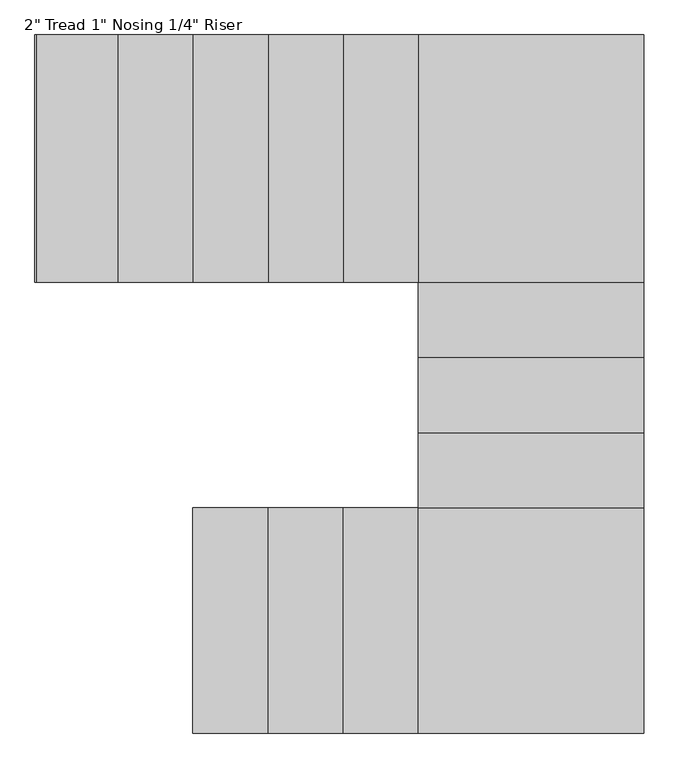
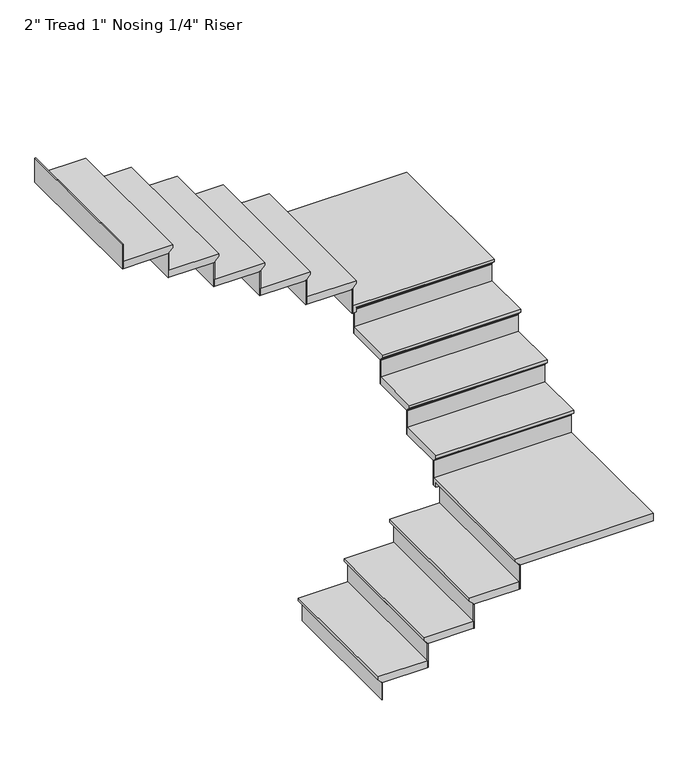
"""IFC4 building model written with IfcOpenShell, lengths in millimetres: stair flight geometry."""

from ifc_helpers import new_model, si_unit, origin, place, context, project, spatial, faceted_brep, source, transform, mapped, element, save


def stair_flight_3451e034(model_context):
    return source(origin(), model_context, "Body", "Brep", [
        faceted_brep([(938.5174794, -182.0870507, 3350.6833333), (938.5174794, -182.0870507, 3369.7333333), (938.5174794, 732.3129493, 3369.7333333), (938.5174794, 732.3129493, 3350.6833333), (963.9174794, -182.0870507, 3325.2833333), (963.9174794, 732.3129493, 3325.2833333), (1268.7174794, -182.0870507, 3369.7333333), (1268.7174794, 732.3129493, 3369.7333333), (963.9174794, 732.3129493, 3318.9333333), (1268.7174794, 732.3129493, 3318.9333333), (1268.7174794, -182.0870507, 3318.9333333), (963.9174794, -182.0870507, 3318.9333333)], [[[0, 1, 2, 3]], [[4, 0, 3, 5]], [[2, 1, 6, 7]], [[8, 9, 10, 11]], [[2, 7, 9, 8, 5, 3]], [[8, 11, 4, 5]], [[6, 1, 0, 4, 11, 10]], [[7, 6, 10, 9]]]),
        faceted_brep([(963.9174794, -182.0870507, 3318.9333333), (963.9174794, -182.0870507, 3200.4), (970.2674794, -182.0870507, 3200.4), (970.2674794, -182.0870507, 3318.9333333), (963.9174794, 732.3129493, 3318.9333333), (970.2674794, 732.3129493, 3318.9333333), (970.2674794, 732.3129493, 3200.4), (963.9174794, 732.3129493, 3200.4)], [[[0, 1, 2, 3]], [[4, 5, 6, 7]], [[1, 0, 4, 7]], [[2, 1, 7, 6]], [[3, 2, 6, 5]], [[0, 3, 5, 4]]]),
        faceted_brep([(1268.7174794, -182.0870507, 3488.2666667), (1268.7174794, -182.0870507, 3318.9333333), (1275.0674794, -182.0870507, 3318.9333333), (1275.0674794, -182.0870507, 3488.2666667), (1268.7174794, 732.3129493, 3488.2666667), (1275.0674794, 732.3129493, 3488.2666667), (1275.0674794, 732.3129493, 3318.9333333), (1268.7174794, 732.3129493, 3318.9333333)], [[[0, 1, 2, 3]], [[4, 5, 6, 7]], [[1, 0, 4, 7]], [[2, 1, 7, 6]], [[3, 2, 6, 5]], [[0, 3, 5, 4]]]),
        faceted_brep([(1243.3174794, 732.3129493, 3539.0666667), (1243.3174794, -182.0870507, 3539.0666667), (1573.5174794, -182.0870507, 3539.0666667), (1573.5174794, 732.3129493, 3539.0666667), (1268.7174794, 732.3129493, 3488.2666667), (1573.5174794, 732.3129493, 3488.2666667), (1573.5174794, -182.0870507, 3488.2666667), (1268.7174794, -182.0870507, 3488.2666667), (1268.7174794, 732.3129493, 3494.6166667), (1243.3174794, 732.3129493, 3520.0166667), (1268.7174794, -182.0870507, 3494.6166667), (1243.3174794, -182.0870507, 3520.0166667)], [[[0, 1, 2, 3]], [[4, 5, 6, 7]], [[0, 3, 5, 4, 8, 9]], [[4, 7, 10, 8]], [[2, 1, 11, 10, 7, 6]], [[3, 2, 6, 5]], [[11, 1, 0, 9]], [[10, 11, 9, 8]]]),
        faceted_brep([(1573.5174794, -182.0870507, 3657.6), (1573.5174794, -182.0870507, 3488.2666667), (1579.8674794, -182.0870507, 3488.2666667), (1579.8674794, -182.0870507, 3657.6), (1573.5174794, 732.3129493, 3657.6), (1579.8674794, 732.3129493, 3657.6), (1579.8674794, 732.3129493, 3488.2666667), (1573.5174794, 732.3129493, 3488.2666667)], [[[0, 1, 2, 3]], [[4, 5, 6, 7]], [[1, 0, 4, 7]], [[2, 1, 7, 6]], [[3, 2, 6, 5]], [[0, 3, 5, 4]]]),
        faceted_brep([(1548.1174794, 732.3129493, 3708.4), (1548.1174794, -182.0870507, 3708.4), (1878.3174794, -182.0870507, 3708.4), (1878.3174794, 732.3129493, 3708.4), (1573.5174794, 732.3129493, 3657.6), (1878.3174794, 732.3129493, 3657.6), (1878.3174794, -182.0870507, 3657.6), (1573.5174794, -182.0870507, 3657.6), (1573.5174794, 732.3129493, 3663.95), (1548.1174794, 732.3129493, 3689.35), (1573.5174794, -182.0870507, 3663.95), (1548.1174794, -182.0870507, 3689.35)], [[[0, 1, 2, 3]], [[4, 5, 6, 7]], [[0, 3, 5, 4, 8, 9]], [[4, 7, 10, 8]], [[2, 1, 11, 10, 7, 6]], [[3, 2, 6, 5]], [[11, 1, 0, 9]], [[10, 11, 9, 8]]]),
        faceted_brep([(1878.3174794, -182.0870507, 3826.9333333), (1878.3174794, -182.0870507, 3657.6), (1884.6674794, -182.0870507, 3657.6), (1884.6674794, -182.0870507, 3826.9333333), (1878.3174794, 732.3129493, 3826.9333333), (1884.6674794, 732.3129493, 3826.9333333), (1884.6674794, 732.3129493, 3657.6), (1878.3174794, 732.3129493, 3657.6)], [[[0, 1, 2, 3]], [[4, 5, 6, 7]], [[1, 0, 4, 7]], [[2, 1, 7, 6]], [[3, 2, 6, 5]], [[0, 3, 5, 4]]]),
        faceted_brep([(2767.3174794, -182.0870507, 3877.7333333), (2767.3174794, 757.7129493, 3877.7333333), (1852.9174794, 757.7129493, 3877.7333333), (1852.9174794, -182.0870507, 3877.7333333), (1852.9174794, 732.3129493, 3826.9333333), (1852.9174794, 757.7129493, 3826.9333333), (2767.3174794, 757.7129493, 3826.9333333), (2767.3174794, -182.0870507, 3826.9333333), (1878.3174794, -182.0870507, 3826.9333333), (1878.3174794, 732.3129493, 3826.9333333), (1852.9174794, 732.3129493, 3858.6833333), (1852.9174794, -182.0870507, 3858.6833333), (1878.3174794, 732.3129493, 3833.2833333), (1878.3174794, -182.0870507, 3833.2833333)], [[[0, 1, 2, 3]], [[4, 5, 6, 7, 8, 9]], [[3, 2, 5, 4, 10, 11]], [[4, 9, 12, 10]], [[9, 8, 13, 12]], [[0, 3, 11, 13, 8, 7]], [[1, 0, 7, 6]], [[2, 1, 6, 5]], [[13, 11, 10, 12]]]),
        faceted_brep([(2767.3174794, 757.7129493, 3996.2666667), (2767.3174794, 757.7129493, 3826.9333333), (2767.3174794, 764.0629493, 3826.9333333), (2767.3174794, 764.0629493, 3996.2666667), (1852.9174794, 757.7129493, 3996.2666667), (1852.9174794, 764.0629493, 3996.2666667), (1852.9174794, 764.0629493, 3826.9333333), (1852.9174794, 757.7129493, 3826.9333333)], [[[0, 1, 2, 3]], [[4, 5, 6, 7]], [[1, 0, 4, 7]], [[2, 1, 7, 6]], [[3, 2, 6, 5]], [[0, 3, 5, 4]]]),
        faceted_brep([(1852.9174794, 732.3129493, 4047.0666667), (2767.3174794, 732.3129493, 4047.0666667), (2767.3174794, 1062.5129493, 4047.0666667), (1852.9174794, 1062.5129493, 4047.0666667), (1852.9174794, 757.7129493, 3996.2666667), (1852.9174794, 1062.5129493, 3996.2666667), (2767.3174794, 1062.5129493, 3996.2666667), (2767.3174794, 757.7129493, 3996.2666667), (1852.9174794, 757.7129493, 4002.6166667), (1852.9174794, 732.3129493, 4028.0166667), (2767.3174794, 757.7129493, 4002.6166667), (2767.3174794, 732.3129493, 4028.0166667)], [[[0, 1, 2, 3]], [[4, 5, 6, 7]], [[0, 3, 5, 4, 8, 9]], [[4, 7, 10, 8]], [[2, 1, 11, 10, 7, 6]], [[3, 2, 6, 5]], [[11, 1, 0, 9]], [[10, 11, 9, 8]]]),
        faceted_brep([(2767.3174794, 1062.5129493, 4165.6), (2767.3174794, 1062.5129493, 3996.2666667), (2767.3174794, 1068.8629493, 3996.2666667), (2767.3174794, 1068.8629493, 4165.6), (1852.9174794, 1062.5129493, 4165.6), (1852.9174794, 1068.8629493, 4165.6), (1852.9174794, 1068.8629493, 3996.2666667), (1852.9174794, 1062.5129493, 3996.2666667)], [[[0, 1, 2, 3]], [[4, 5, 6, 7]], [[1, 0, 4, 7]], [[2, 1, 7, 6]], [[3, 2, 6, 5]], [[0, 3, 5, 4]]]),
        faceted_brep([(1852.9174794, 1037.1129493, 4216.4), (2767.3174794, 1037.1129493, 4216.4), (2767.3174794, 1367.3129493, 4216.4), (1852.9174794, 1367.3129493, 4216.4), (1852.9174794, 1062.5129493, 4165.6), (1852.9174794, 1367.3129493, 4165.6), (2767.3174794, 1367.3129493, 4165.6), (2767.3174794, 1062.5129493, 4165.6), (1852.9174794, 1062.5129493, 4171.95), (1852.9174794, 1037.1129493, 4197.35), (2767.3174794, 1062.5129493, 4171.95), (2767.3174794, 1037.1129493, 4197.35)], [[[0, 1, 2, 3]], [[4, 5, 6, 7]], [[0, 3, 5, 4, 8, 9]], [[4, 7, 10, 8]], [[2, 1, 11, 10, 7, 6]], [[3, 2, 6, 5]], [[11, 1, 0, 9]], [[10, 11, 9, 8]]]),
        faceted_brep([(2767.3174794, 1367.3129493, 4334.9333333), (2767.3174794, 1367.3129493, 4165.6), (2767.3174794, 1373.6629493, 4165.6), (2767.3174794, 1373.6629493, 4334.9333333), (1852.9174794, 1367.3129493, 4334.9333333), (1852.9174794, 1373.6629493, 4334.9333333), (1852.9174794, 1373.6629493, 4165.6), (1852.9174794, 1367.3129493, 4165.6)], [[[0, 1, 2, 3]], [[4, 5, 6, 7]], [[1, 0, 4, 7]], [[2, 1, 7, 6]], [[3, 2, 6, 5]], [[0, 3, 5, 4]]]),
        faceted_brep([(1852.9174794, 1341.9129493, 4385.7333333), (2767.3174794, 1341.9129493, 4385.7333333), (2767.3174794, 1672.1129493, 4385.7333333), (1852.9174794, 1672.1129493, 4385.7333333), (1852.9174794, 1367.3129493, 4334.9333333), (1852.9174794, 1672.1129493, 4334.9333333), (2767.3174794, 1672.1129493, 4334.9333333), (2767.3174794, 1367.3129493, 4334.9333333), (1852.9174794, 1367.3129493, 4341.2833333), (1852.9174794, 1341.9129493, 4366.6833333), (2767.3174794, 1367.3129493, 4341.2833333), (2767.3174794, 1341.9129493, 4366.6833333)], [[[0, 1, 2, 3]], [[4, 5, 6, 7]], [[0, 3, 5, 4, 8, 9]], [[4, 7, 10, 8]], [[2, 1, 11, 10, 7, 6]], [[3, 2, 6, 5]], [[11, 1, 0, 9]], [[10, 11, 9, 8]]]),
        faceted_brep([(2767.3174794, 1672.1129493, 4504.2666667), (2767.3174794, 1672.1129493, 4334.9333333), (2767.3174794, 1678.4629493, 4334.9333333), (2767.3174794, 1678.4629493, 4504.2666667), (1852.9174794, 1672.1129493, 4504.2666667), (1852.9174794, 1678.4629493, 4504.2666667), (1852.9174794, 1678.4629493, 4334.9333333), (1852.9174794, 1672.1129493, 4334.9333333)], [[[0, 1, 2, 3]], [[4, 5, 6, 7]], [[1, 0, 4, 7]], [[2, 1, 7, 6]], [[3, 2, 6, 5]], [[0, 3, 5, 4]]]),
        faceted_brep([(2767.3174794, 2650.0129493, 4555.0666667), (1827.5174794, 2650.0129493, 4555.0666667), (1827.5174794, 1646.7129493, 4555.0666667), (2767.3174794, 1646.7129493, 4555.0666667), (1852.9174794, 1646.7129493, 4504.2666667), (1827.5174794, 1646.7129493, 4504.2666667), (1827.5174794, 2650.0129493, 4504.2666667), (2767.3174794, 2650.0129493, 4504.2666667), (2767.3174794, 1672.1129493, 4504.2666667), (1852.9174794, 1672.1129493, 4504.2666667), (1852.9174794, 1646.7129493, 4536.0166667), (2767.3174794, 1646.7129493, 4536.0166667), (1852.9174794, 1672.1129493, 4510.6166667), (2767.3174794, 1672.1129493, 4510.6166667)], [[[0, 1, 2, 3]], [[4, 5, 6, 7, 8, 9]], [[3, 2, 5, 4, 10, 11]], [[4, 9, 12, 10]], [[9, 8, 13, 12]], [[0, 3, 11, 13, 8, 7]], [[1, 0, 7, 6]], [[2, 1, 6, 5]], [[13, 11, 10, 12]]]),
        faceted_brep([(1827.5174794, 2650.0129493, 4673.6), (1827.5174794, 2650.0129493, 4504.2666667), (1821.1674794, 2650.0129493, 4504.2666667), (1821.1674794, 2650.0129493, 4673.6), (1827.5174794, 1646.7129493, 4673.6), (1821.1674794, 1646.7129493, 4673.6), (1821.1674794, 1646.7129493, 4504.2666667), (1827.5174794, 1646.7129493, 4504.2666667)], [[[0, 1, 2, 3]], [[4, 5, 6, 7]], [[1, 0, 4, 7]], [[2, 1, 7, 6]], [[3, 2, 6, 5]], [[0, 3, 5, 4]]]),
        faceted_brep([(1852.9174794, 1646.7129493, 4724.4), (1852.9174794, 2650.0129493, 4724.4), (1522.7174794, 2650.0129493, 4724.4), (1522.7174794, 1646.7129493, 4724.4), (1827.5174794, 1646.7129493, 4673.6), (1522.7174794, 1646.7129493, 4673.6), (1522.7174794, 2650.0129493, 4673.6), (1827.5174794, 2650.0129493, 4673.6), (1827.5174794, 1646.7129493, 4679.95), (1852.9174794, 1646.7129493, 4705.35), (1827.5174794, 2650.0129493, 4679.95), (1852.9174794, 2650.0129493, 4705.35)], [[[0, 1, 2, 3]], [[4, 5, 6, 7]], [[0, 3, 5, 4, 8, 9]], [[4, 7, 10, 8]], [[2, 1, 11, 10, 7, 6]], [[3, 2, 6, 5]], [[11, 1, 0, 9]], [[10, 11, 9, 8]]]),
        faceted_brep([(1522.7174794, 2650.0129493, 4842.9333333), (1522.7174794, 2650.0129493, 4673.6), (1516.3674794, 2650.0129493, 4673.6), (1516.3674794, 2650.0129493, 4842.9333333), (1522.7174794, 1646.7129493, 4842.9333333), (1516.3674794, 1646.7129493, 4842.9333333), (1516.3674794, 1646.7129493, 4673.6), (1522.7174794, 1646.7129493, 4673.6)], [[[0, 1, 2, 3]], [[4, 5, 6, 7]], [[1, 0, 4, 7]], [[2, 1, 7, 6]], [[3, 2, 6, 5]], [[0, 3, 5, 4]]]),
        faceted_brep([(1548.1174794, 1646.7129493, 4893.7333333), (1548.1174794, 2650.0129493, 4893.7333333), (1217.9174794, 2650.0129493, 4893.7333333), (1217.9174794, 1646.7129493, 4893.7333333), (1522.7174794, 1646.7129493, 4842.9333333), (1217.9174794, 1646.7129493, 4842.9333333), (1217.9174794, 2650.0129493, 4842.9333333), (1522.7174794, 2650.0129493, 4842.9333333), (1522.7174794, 1646.7129493, 4849.2833333), (1548.1174794, 1646.7129493, 4874.6833333), (1522.7174794, 2650.0129493, 4849.2833333), (1548.1174794, 2650.0129493, 4874.6833333)], [[[0, 1, 2, 3]], [[4, 5, 6, 7]], [[0, 3, 5, 4, 8, 9]], [[4, 7, 10, 8]], [[2, 1, 11, 10, 7, 6]], [[3, 2, 6, 5]], [[11, 1, 0, 9]], [[10, 11, 9, 8]]]),
        faceted_brep([(1217.9174794, 2650.0129493, 5012.2666667), (1217.9174794, 2650.0129493, 4842.9333333), (1211.5674794, 2650.0129493, 4842.9333333), (1211.5674794, 2650.0129493, 5012.2666667), (1217.9174794, 1646.7129493, 5012.2666667), (1211.5674794, 1646.7129493, 5012.2666667), (1211.5674794, 1646.7129493, 4842.9333333), (1217.9174794, 1646.7129493, 4842.9333333)], [[[0, 1, 2, 3]], [[4, 5, 6, 7]], [[1, 0, 4, 7]], [[2, 1, 7, 6]], [[3, 2, 6, 5]], [[0, 3, 5, 4]]]),
        faceted_brep([(1243.3174794, 1646.7129493, 5063.0666667), (1243.3174794, 2650.0129493, 5063.0666667), (913.1174794, 2650.0129493, 5063.0666667), (913.1174794, 1646.7129493, 5063.0666667), (1217.9174794, 1646.7129493, 5012.2666667), (913.1174794, 1646.7129493, 5012.2666667), (913.1174794, 2650.0129493, 5012.2666667), (1217.9174794, 2650.0129493, 5012.2666667), (1217.9174794, 1646.7129493, 5018.6166667), (1243.3174794, 1646.7129493, 5044.0166667), (1217.9174794, 2650.0129493, 5018.6166667), (1243.3174794, 2650.0129493, 5044.0166667)], [[[0, 1, 2, 3]], [[4, 5, 6, 7]], [[0, 3, 5, 4, 8, 9]], [[4, 7, 10, 8]], [[2, 1, 11, 10, 7, 6]], [[3, 2, 6, 5]], [[11, 1, 0, 9]], [[10, 11, 9, 8]]]),
        faceted_brep([(913.1174794, 2650.0129493, 5181.6), (913.1174794, 2650.0129493, 5012.2666667), (906.7674794, 2650.0129493, 5012.2666667), (906.7674794, 2650.0129493, 5181.6), (913.1174794, 1646.7129493, 5181.6), (906.7674794, 1646.7129493, 5181.6), (906.7674794, 1646.7129493, 5012.2666667), (913.1174794, 1646.7129493, 5012.2666667)], [[[0, 1, 2, 3]], [[4, 5, 6, 7]], [[1, 0, 4, 7]], [[2, 1, 7, 6]], [[3, 2, 6, 5]], [[0, 3, 5, 4]]]),
        faceted_brep([(938.5174794, 1646.7129493, 5232.4), (938.5174794, 2650.0129493, 5232.4), (608.3174794, 2650.0129493, 5232.4), (608.3174794, 1646.7129493, 5232.4), (913.1174794, 1646.7129493, 5181.6), (608.3174794, 1646.7129493, 5181.6), (608.3174794, 2650.0129493, 5181.6), (913.1174794, 2650.0129493, 5181.6), (913.1174794, 1646.7129493, 5187.95), (938.5174794, 1646.7129493, 5213.35), (913.1174794, 2650.0129493, 5187.95), (938.5174794, 2650.0129493, 5213.35)], [[[0, 1, 2, 3]], [[4, 5, 6, 7]], [[0, 3, 5, 4, 8, 9]], [[4, 7, 10, 8]], [[2, 1, 11, 10, 7, 6]], [[3, 2, 6, 5]], [[11, 1, 0, 9]], [[10, 11, 9, 8]]]),
        faceted_brep([(608.3174794, 2650.0129493, 5350.9333333), (608.3174794, 2650.0129493, 5181.6), (601.9674794, 2650.0129493, 5181.6), (601.9674794, 2650.0129493, 5350.9333333), (608.3174794, 1646.7129493, 5350.9333333), (601.9674794, 1646.7129493, 5350.9333333), (601.9674794, 1646.7129493, 5181.6), (608.3174794, 1646.7129493, 5181.6)], [[[0, 1, 2, 3]], [[4, 5, 6, 7]], [[1, 0, 4, 7]], [[2, 1, 7, 6]], [[3, 2, 6, 5]], [[0, 3, 5, 4]]]),
        faceted_brep([(303.5174794, 2650.0129493, 5520.2666667), (303.5174794, 2650.0129493, 5350.9333333), (297.1674794, 2650.0129493, 5350.9333333), (297.1674794, 2650.0129493, 5520.2666667), (303.5174794, 1646.7129493, 5520.2666667), (297.1674794, 1646.7129493, 5520.2666667), (297.1674794, 1646.7129493, 5350.9333333), (303.5174794, 1646.7129493, 5350.9333333)], [[[0, 1, 2, 3]], [[4, 5, 6, 7]], [[1, 0, 4, 7]], [[2, 1, 7, 6]], [[3, 2, 6, 5]], [[0, 3, 5, 4]]]),
        faceted_brep([(633.7174794, 1646.7129493, 5401.7333333), (633.7174794, 2650.0129493, 5401.7333333), (303.5174794, 2650.0129493, 5401.7333333), (303.5174794, 1646.7129493, 5401.7333333), (608.3174794, 1646.7129493, 5350.9333333), (303.5174794, 1646.7129493, 5350.9333333), (303.5174794, 2650.0129493, 5350.9333333), (608.3174794, 2650.0129493, 5350.9333333), (608.3174794, 1646.7129493, 5357.2833333), (633.7174794, 1646.7129493, 5382.6833333), (608.3174794, 2650.0129493, 5357.2833333), (633.7174794, 2650.0129493, 5382.6833333)], [[[0, 1, 2, 3]], [[4, 5, 6, 7]], [[0, 3, 5, 4, 8, 9]], [[4, 7, 10, 8]], [[2, 1, 11, 10, 7, 6]], [[3, 2, 6, 5]], [[11, 1, 0, 9]], [[10, 11, 9, 8]]]),
    ])


if __name__ == "__main__":
    model = new_model("IFC4")
    model_context = context("Model", 3, world=origin())
    ifc_project = project(units=[si_unit("LENGTHUNIT", "METRE", prefix="MILLI")], contexts=[model_context])
    site = spatial("IfcSite", under=ifc_project)
    building = spatial("IfcBuilding", under=site)
    placement = place(None, origin())
    stair_flight_shape = stair_flight_3451e034(model_context)
    element("IfcStairFlight", 1, ObjectType="2\" Tread 1\" Nosing 1/4\" Riser", at=placement, inside=building, context=model_context, shape_type="MappedRepresentation", body=[
        mapped(stair_flight_shape, transform((0.0, 0.0, 0.0), x_axis=(1.0, 0.0, 0.0), y_axis=(0.0, 1.0, 0.0), z_axis=(0.0, 0.0, 1.0))),
    ])
    save(model, "model.ifc")
